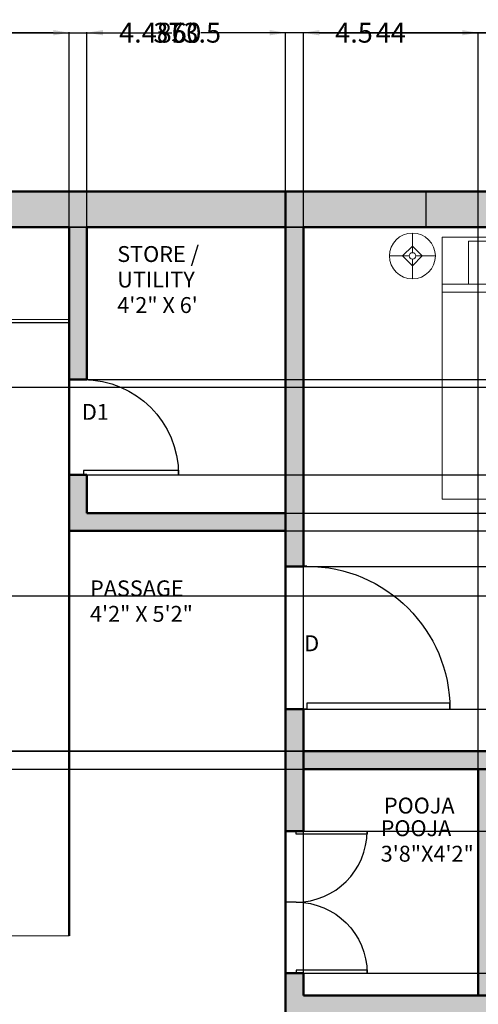
# Model space of a CAD drawing. Units: inches. Extents: x -12 to 887, y 330 to 874.
# Tile 8 of 9: x 605 to 720, y 626 to 874. Entities that reach past the tile are written whole.
import ezdxf

# ---------------------------------------------------------------- set-up
doc = ezdxf.new("R2010")
doc.units = ezdxf.units.IN
doc.header["$MEASUREMENT"] = 0
for name, color, linetype, lineweight in [('A-ANNO-DIMS', 2, 'Continuous', 18), ('A-ANNO-TEXT', 3, 'Continuous', 18), ('A-AREA-IDEN', 7, 'Continuous', 18), ('A-DOOR', 4, 'Continuous', 25), ('A-EQPM', 8, 'Continuous', 18), ('A-FLOR-FIXT', 8, 'Continuous', 18), ('A-FURN', 9, 'Continuous', 18), ('A-GLAZ', 4, 'Continuous', 25), ('A-WALL', 7, 'Continuous', 50), ('A-WALL-PATT', 5, 'Continuous', 13)]:
    doc.layers.add(name, color=color, linetype=linetype, lineweight=lineweight)
doc.styles.get("Standard").update_dxf_attribs({"font": 'arial.ttf'})
doc.dimstyles.get("Standard").update_dxf_attribs({"dimtxt": 5, "dimasz": 4, "dimexe": 0.18, "dimexo": 0.0625, "dimgap": 0.09, "dimtad": 0, "dimtih": 1, "dimtoh": 1, "dimdec": 1, "dimzin": 0, "dimdsep": 46, "dimlunit": 4, "dimtxsty": 'Standard', "dimcen": 0.09, "dimadec": 0, "dimazin": 0, "dimtfac": 1, "dimtdec": 1, "dimtofl": 0, "dimtmove": 0, "dimatfit": 3, "dimfxl": 1, "dimtolj": 1, "dimtzin": 0, "dimarcsym": 0})

# ---------------------------------------------------------------- blocks, each defined once
blk = doc.blocks.new('Refrigerator-2 door - 36 in top')
for p, q in [((0, -26.999999), (36, -26.999999)), ((11, -27.999999), (11, -28.999999)), ((12, -26.999999), (12, -28.999999)), ((13, -28.999999), (13, -27.999999)), ((11, -28.999999), (13, -28.999999))]:
    blk.add_line(p, q)
blk.add_lwpolyline([(0, -27.999999), (0, 0), (36, 0), (36, -27.999999)], close=True)
blk = doc.blocks.new('*U5')
for p, q in [((0, 0), (0, -6)), ((40, 0), (40, -6))]:
    blk.add_line(p, q)
blk.add_lwpolyline([(0, 0), (0, 40), (1.75, 40), (1.75, 0)], close=True)
blk.add_arc((0, 0), 40, 0, 90)
blk = doc.blocks.new('Bed - Queen')
for p, q in [((0, -80.00003), (0, 0)), ((0, 0), (59.99999, 0)), ((59.99999, 0), (59.99999, -80.00003)), ((7.99999, -1.2), (28.79998, -1.2)), ((7.99999, -14.4), (7.99999, -1.2)), ((28.79998, -1.2), (28.79998, -14.4)), ((31.19999, -1.2), (51.99999, -1.2)), ((31.19999, -14.4), (31.19999, -1.2)), ((51.99999, -1.2), (51.99999, -16.4)), ((0, -14.4), (44.8, -14.4)), ((59.99999, -29.6), (44.8, -14.4)), ((44.8, -14.4), (44.8, -29.6)), ((44.8, -16.8), (0, -16.8)), ((51.99999, -16.4), (46.79936, -16.4)), ((44.8, -29.6), (59.99999, -29.6)), ((59.99999, -80.00003), (0, -80.00003))]:
    blk.add_line(p, q)
blk = doc.blocks.new('Lamp - Table')
for p, q in [((0, 7), (0, 1)), ((-1, 0), (-7, 0)), ((0, 3), (-3, 0)), ((-3, 0), (0, -3)), ((3, 0), (0, 3)), ((0, -3), (3, 0)), ((1, 0), (7, 0)), ((0, -1), (0, -7))]:
    blk.add_line(p, q)
for radius in [7, 1]:
    blk.add_circle((0, 0), radius)
blk = doc.blocks.new('*D64')
at = {"layer": 'A-ANNO-DIMS', "color": 0, "lineweight": -2, "transparency": 16777216}
for p, q in [((383.99, 685.16), (873.75, 685.16)), ((873.57, 681.16), (873.57, 628.55)), ((873.57, 570.66), (873.57, 623.27)), ((383.99, 566.66), (873.75, 566.66))]:
    blk.add_line(p, q, dxfattribs=at)
at = {"layer": 'A-ANNO-DIMS', "color": 0, "transparency": 16777216}
for points in [[(872.9, 681.16), (874.24, 681.16), (873.57, 685.16)], [(872.9, 570.66), (874.24, 570.66), (873.57, 566.66)]]:
    blk.add_solid(points, dxfattribs=at)
at = {"layer": 'Defpoints', "color": 0, "transparency": 16777216}
for p in [(383.93, 685.16), (873.57, 685.16), (383.93, 566.66)]:
    blk.add_point(p, dxfattribs=at)
at = {"layer": 'A-ANNO-DIMS', "color": 0, "transparency": 16777216, "insert": (873.57, 625.91), "char_height": 5, "attachment_point": 5}
blk.add_mtext('\\A1;118.5', dxfattribs=at)
blk = doc.blocks.new('*D65')
at = {"layer": 'A-ANNO-DIMS', "color": 0, "lineweight": -2, "transparency": 16777216}
for p, q in [((873.57, 693.66), (873.57, 697.66)), ((873.57, 697.66), (877.57, 697.66)), ((383.99, 689.66), (873.75, 689.66)), ((383.99, 685.16), (873.75, 685.16)), ((873.57, 681.16), (873.57, 677.16))]:
    blk.add_line(p, q, dxfattribs=at)
at = {"layer": 'A-ANNO-DIMS', "color": 0, "transparency": 16777216}
for points in [[(872.9, 693.66), (874.24, 693.66), (873.57, 689.66)], [(872.9, 681.16), (874.24, 681.16), (873.57, 685.16)]]:
    blk.add_solid(points, dxfattribs=at)
at = {"layer": 'Defpoints', "color": 0, "transparency": 16777216}
for p in [(383.93, 689.66), (873.57, 689.66), (383.93, 685.16)]:
    blk.add_point(p, dxfattribs=at)
at = {"layer": 'A-ANNO-DIMS', "color": 0, "transparency": 16777216, "insert": (882.33, 697.66), "char_height": 5, "attachment_point": 5}
blk.add_mtext('\\A1;4.5', dxfattribs=at)
blk = doc.blocks.new('*D66')
at = {"layer": 'A-ANNO-DIMS', "color": 0, "lineweight": -2, "transparency": 16777216}
for p, q in [((383.99, 821.66), (873.75, 821.66)), ((873.57, 817.66), (873.57, 758.31)), ((873.57, 693.66), (873.57, 753.02)), ((383.99, 689.66), (873.75, 689.66))]:
    blk.add_line(p, q, dxfattribs=at)
at = {"layer": 'A-ANNO-DIMS', "color": 0, "transparency": 16777216}
for points in [[(872.9, 817.66), (874.24, 817.66), (873.57, 821.66)], [(872.9, 693.66), (874.24, 693.66), (873.57, 689.66)]]:
    blk.add_solid(points, dxfattribs=at)
at = {"layer": 'Defpoints', "color": 0, "transparency": 16777216}
for p in [(383.93, 821.66), (873.57, 821.66), (383.93, 689.66)]:
    blk.add_point(p, dxfattribs=at)
at = {"layer": 'A-ANNO-DIMS', "color": 0, "transparency": 16777216, "insert": (873.57, 755.66), "char_height": 5, "attachment_point": 5}
blk.add_mtext('\\A1;132', dxfattribs=at)
blk = doc.blocks.new('*D83')
at = {"layer": 'A-ANNO-DIMS', "color": 0, "lineweight": -2, "transparency": 16777216}
for p, q in [((460.07, 830.72), (460.07, 870.84)), ((464.07, 870.66), (638.28, 870.66)), ((829.57, 870.66), (655.36, 870.66)), ((833.57, 830.72), (833.57, 870.84))]:
    blk.add_line(p, q, dxfattribs=at)
at = {"layer": 'A-ANNO-DIMS', "color": 0, "transparency": 16777216}
for points in [[(464.07, 871.33), (464.07, 869.99), (460.07, 870.66)], [(829.57, 871.33), (829.57, 869.99), (833.57, 870.66)]]:
    blk.add_solid(points, dxfattribs=at)
at = {"layer": 'Defpoints', "color": 0, "transparency": 16777216}
for p in [(833.57, 870.66), (460.07, 830.66), (833.57, 830.66)]:
    blk.add_point(p, dxfattribs=at)
at = {"layer": 'A-ANNO-DIMS', "color": 0, "transparency": 16777216, "insert": (646.82, 870.66), "char_height": 5, "attachment_point": 5}
blk.add_mtext('\\A1;373.5', dxfattribs=at)
blk = doc.blocks.new('*D87')
at = {"layer": 'A-ANNO-DIMS', "color": 0, "lineweight": -2, "transparency": 16777216}
for p, q in [((493.07, 821.72), (493.07, 870.84)), ((497.07, 870.66), (545.32, 870.66)), ((613.08, 870.66), (564.83, 870.66)), ((617.08, 821.7), (617.08, 870.84))]:
    blk.add_line(p, q, dxfattribs=at)
at = {"layer": 'A-ANNO-DIMS', "color": 0, "transparency": 16777216}
for points in [[(497.07, 871.33), (497.07, 869.99), (493.07, 870.66)], [(613.08, 871.33), (613.08, 869.99), (617.08, 870.66)]]:
    blk.add_solid(points, dxfattribs=at)
at = {"layer": 'Defpoints', "color": 0, "transparency": 16777216}
for p in [(617.08, 870.66), (493.07, 821.66), (617.08, 821.64)]:
    blk.add_point(p, dxfattribs=at)
at = {"layer": 'A-ANNO-DIMS', "color": 0, "transparency": 16777216, "insert": (555.08, 870.66), "char_height": 5, "attachment_point": 5}
blk.add_mtext('\\A1;124.01', dxfattribs=at)
blk = doc.blocks.new('*D88')
at = {"layer": 'A-ANNO-DIMS', "color": 0, "lineweight": -2, "transparency": 16777216}
for p, q in [((613.08, 870.66), (609.08, 870.66)), ((617.08, 821.7), (617.08, 870.84)), ((621.57, 821.72), (621.57, 870.84)), ((625.57, 870.66), (629.57, 870.66))]:
    blk.add_line(p, q, dxfattribs=at)
at = {"layer": 'A-ANNO-DIMS', "color": 0, "transparency": 16777216}
for points in [[(613.08, 871.33), (613.08, 869.99), (617.08, 870.66)], [(625.57, 871.33), (625.57, 869.99), (621.57, 870.66)]]:
    blk.add_solid(points, dxfattribs=at)
at = {"layer": 'Defpoints', "color": 0, "transparency": 16777216}
for p in [(621.57, 870.66), (617.08, 821.64), (621.57, 821.66)]:
    blk.add_point(p, dxfattribs=at)
at = {"layer": 'A-ANNO-DIMS', "color": 0, "transparency": 16777216, "insert": (638.19, 870.66), "char_height": 5, "attachment_point": 5}
blk.add_mtext('\\A1;4.486', dxfattribs=at)
blk = doc.blocks.new('*D89')
at = {"layer": 'A-ANNO-DIMS', "color": 0, "lineweight": -2, "transparency": 16777216}
for p, q in [((621.57, 821.72), (621.57, 870.84)), ((625.57, 870.66), (642.91, 870.66)), ((667.57, 870.66), (650.23, 870.66)), ((671.57, 821.72), (671.57, 870.84))]:
    blk.add_line(p, q, dxfattribs=at)
at = {"layer": 'A-ANNO-DIMS', "color": 0, "transparency": 16777216}
for points in [[(625.57, 871.33), (625.57, 869.99), (621.57, 870.66)], [(667.57, 871.33), (667.57, 869.99), (671.57, 870.66)]]:
    blk.add_solid(points, dxfattribs=at)
at = {"layer": 'Defpoints', "color": 0, "transparency": 16777216}
for p in [(671.57, 870.66), (621.57, 821.66), (671.57, 821.66)]:
    blk.add_point(p, dxfattribs=at)
at = {"layer": 'A-ANNO-DIMS', "color": 0, "transparency": 16777216, "insert": (646.57, 870.66), "char_height": 5, "attachment_point": 5}
blk.add_mtext('\\A1;50', dxfattribs=at)
blk = doc.blocks.new('*D90')
at = {"layer": 'A-ANNO-DIMS', "color": 0, "lineweight": -2, "transparency": 16777216}
for p, q in [((667.57, 870.66), (663.57, 870.66)), ((671.57, 821.72), (671.57, 870.84)), ((676.07, 821.72), (676.07, 870.84)), ((680.07, 870.66), (684.07, 870.66))]:
    blk.add_line(p, q, dxfattribs=at)
at = {"layer": 'A-ANNO-DIMS', "color": 0, "transparency": 16777216}
for points in [[(667.57, 871.33), (667.57, 869.99), (671.57, 870.66)], [(680.07, 871.33), (680.07, 869.99), (676.07, 870.66)]]:
    blk.add_solid(points, dxfattribs=at)
at = {"layer": 'Defpoints', "color": 0, "transparency": 16777216}
for p in [(676.07, 870.66), (671.57, 821.66), (676.07, 821.66)]:
    blk.add_point(p, dxfattribs=at)
at = {"layer": 'A-ANNO-DIMS', "color": 0, "transparency": 16777216, "insert": (688.83, 870.66), "char_height": 5, "attachment_point": 5}
blk.add_mtext('\\A1;4.5', dxfattribs=at)
blk = doc.blocks.new('*D91')
at = {"layer": 'A-ANNO-DIMS', "color": 0, "lineweight": -2, "transparency": 16777216}
for p, q in [((676.07, 821.72), (676.07, 870.84)), ((680.07, 870.66), (733.69, 870.66)), ((798.07, 870.66), (744.44, 870.66)), ((802.07, 821.72), (802.07, 870.84))]:
    blk.add_line(p, q, dxfattribs=at)
at = {"layer": 'A-ANNO-DIMS', "color": 0, "transparency": 16777216}
for points in [[(680.07, 871.33), (680.07, 869.99), (676.07, 870.66)], [(798.07, 871.33), (798.07, 869.99), (802.07, 870.66)]]:
    blk.add_solid(points, dxfattribs=at)
at = {"layer": 'Defpoints', "color": 0, "transparency": 16777216}
for p in [(802.07, 870.66), (676.07, 821.66), (802.07, 821.66)]:
    blk.add_point(p, dxfattribs=at)
at = {"layer": 'A-ANNO-DIMS', "color": 0, "transparency": 16777216, "insert": (739.07, 870.66), "char_height": 5, "attachment_point": 5}
blk.add_mtext('\\A1;126', dxfattribs=at)
blk = doc.blocks.new('*D98')
at = {"layer": 'A-ANNO-DIMS', "color": 0, "lineweight": -2, "transparency": 16777216}
for p, q in [((460.13, 830.66), (873.75, 830.66)), ((873.57, 826.66), (873.57, 604.54)), ((873.57, 377.16), (873.57, 599.28)), ((460.13, 373.16), (873.75, 373.16))]:
    blk.add_line(p, q, dxfattribs=at)
at = {"layer": 'A-ANNO-DIMS', "color": 0, "transparency": 16777216}
for points in [[(872.9, 826.66), (874.24, 826.66), (873.57, 830.66)], [(872.9, 377.16), (874.24, 377.16), (873.57, 373.16)]]:
    blk.add_solid(points, dxfattribs=at)
at = {"layer": 'Defpoints', "color": 0, "transparency": 16777216}
for p in [(460.07, 830.66), (873.57, 830.66), (460.07, 373.16)]:
    blk.add_point(p, dxfattribs=at)
at = {"layer": 'A-ANNO-DIMS', "color": 0, "transparency": 16777216, "insert": (873.57, 601.91), "char_height": 5, "attachment_point": 5}
blk.add_mtext('\\A1;457.5', dxfattribs=at)
blk = doc.blocks.new('*D112')
at = {"layer": 'A-ANNO-DIMS', "color": 0, "lineweight": -2, "transparency": 16777216}
for p, q in [((676.01, 821.66), (1.75, 821.66)), ((1.93, 817.66), (1.93, 758.31)), ((1.93, 693.66), (1.93, 753.02)), ((676.01, 689.66), (1.75, 689.66))]:
    blk.add_line(p, q, dxfattribs=at)
at = {"layer": 'A-ANNO-DIMS', "color": 0, "transparency": 16777216}
for points in [[(1.26, 817.66), (2.59, 817.66), (1.93, 821.66)], [(1.26, 693.66), (2.59, 693.66), (1.93, 689.66)]]:
    blk.add_solid(points, dxfattribs=at)
at = {"layer": 'Defpoints', "color": 0, "transparency": 16777216}
for p in [(1.93, 821.66), (676.07, 821.66), (676.07, 689.66)]:
    blk.add_point(p, dxfattribs=at)
at = {"layer": 'A-ANNO-DIMS', "color": 0, "transparency": 16777216, "insert": (1.93, 755.66), "char_height": 5, "attachment_point": 5}
blk.add_mtext('\\A1;132', dxfattribs=at)
blk = doc.blocks.new('*D113')
at = {"layer": 'A-ANNO-DIMS', "color": 0, "lineweight": -2, "transparency": 16777216}
for p, q in [((676.07, 628.22), (676.07, 870.84)), ((680.07, 870.66), (694.31, 870.66)), ((716.07, 870.66), (701.83, 870.66)), ((720.07, 628.22), (720.07, 870.84))]:
    blk.add_line(p, q, dxfattribs=at)
at = {"layer": 'A-ANNO-DIMS', "color": 0, "transparency": 16777216}
for points in [[(680.07, 871.33), (680.07, 869.99), (676.07, 870.66)], [(716.07, 871.33), (716.07, 869.99), (720.07, 870.66)]]:
    blk.add_solid(points, dxfattribs=at)
at = {"layer": 'Defpoints', "color": 0, "transparency": 16777216}
for p in [(720.07, 870.66), (676.07, 628.16), (720.07, 628.16)]:
    blk.add_point(p, dxfattribs=at)
at = {"layer": 'A-ANNO-DIMS', "color": 0, "transparency": 16777216, "insert": (698.07, 870.66), "char_height": 5, "attachment_point": 5}
blk.add_mtext('\\A1;44', dxfattribs=at)
blk = doc.blocks.new('*D116')
at = {"layer": 'A-ANNO-DIMS', "color": 0, "lineweight": -2, "transparency": 16777216}
for p, q in [((873.57, 753.66), (873.57, 757.66)), ((621.63, 749.66), (873.75, 749.66)), ((617.13, 745.16), (873.75, 745.16)), ((873.57, 741.16), (873.57, 737.16)), ((873.57, 737.16), (869.57, 737.16))]:
    blk.add_line(p, q, dxfattribs=at)
at = {"layer": 'A-ANNO-DIMS', "color": 0, "transparency": 16777216}
for points in [[(872.9, 753.66), (874.24, 753.66), (873.57, 749.66)], [(872.9, 741.16), (874.24, 741.16), (873.57, 745.16)]]:
    blk.add_solid(points, dxfattribs=at)
at = {"layer": 'Defpoints', "color": 0, "transparency": 16777216}
for p in [(621.57, 749.66), (617.07, 745.16), (873.57, 745.16)]:
    blk.add_point(p, dxfattribs=at)
at = {"layer": 'A-ANNO-DIMS', "color": 0, "transparency": 16777216, "insert": (864.81, 737.16), "char_height": 5, "attachment_point": 5}
blk.add_mtext('\\A1;4.5', dxfattribs=at)
blk = doc.blocks.new('*D117')
at = {"layer": 'A-ANNO-DIMS', "color": 0, "lineweight": -2, "transparency": 16777216}
for p, q in [((621.63, 821.66), (873.75, 821.66)), ((873.57, 817.66), (873.57, 788.26)), ((873.57, 753.66), (873.57, 783.06)), ((621.63, 749.66), (873.75, 749.66))]:
    blk.add_line(p, q, dxfattribs=at)
at = {"layer": 'A-ANNO-DIMS', "color": 0, "transparency": 16777216}
for points in [[(872.9, 817.66), (874.24, 817.66), (873.57, 821.66)], [(872.9, 753.66), (874.24, 753.66), (873.57, 749.66)]]:
    blk.add_solid(points, dxfattribs=at)
at = {"layer": 'Defpoints', "color": 0, "transparency": 16777216}
for p in [(621.57, 821.66), (873.57, 821.66), (621.57, 749.66)]:
    blk.add_point(p, dxfattribs=at)
at = {"layer": 'A-ANNO-DIMS', "color": 0, "transparency": 16777216, "insert": (873.57, 785.66), "char_height": 5, "attachment_point": 5}
blk.add_mtext('\\A1;72', dxfattribs=at)
blk = doc.blocks.new('*D122')
at = {"layer": 'A-ANNO-DIMS', "color": 0, "lineweight": -2, "transparency": 16777216}
for p, q in [((671.63, 736.22), (873.75, 736.22)), ((873.57, 732.22), (873.57, 720.87)), ((873.57, 704.22), (873.57, 715.58)), ((671.63, 700.22), (873.75, 700.22))]:
    blk.add_line(p, q, dxfattribs=at)
at = {"layer": 'A-ANNO-DIMS', "color": 0, "transparency": 16777216}
for points in [[(872.9, 732.22), (874.24, 732.22), (873.57, 736.22)], [(872.9, 704.22), (874.24, 704.22), (873.57, 700.22)]]:
    blk.add_solid(points, dxfattribs=at)
at = {"layer": 'Defpoints', "color": 0, "transparency": 16777216}
for p in [(671.57, 736.22), (671.57, 700.22), (873.57, 700.22)]:
    blk.add_point(p, dxfattribs=at)
at = {"layer": 'A-ANNO-DIMS', "color": 0, "transparency": 16777216, "insert": (873.57, 718.22), "char_height": 5, "attachment_point": 5}
blk.add_mtext('\\A1;36', dxfattribs=at)
blk = doc.blocks.new('*D123')
at = {"layer": 'A-ANNO-DIMS', "color": 0, "lineweight": -2, "transparency": 16777216}
for p, q in [((617.13, 783.29), (873.75, 783.29)), ((873.57, 779.29), (873.57, 773.94)), ((873.57, 763.31), (873.57, 768.65)), ((617.13, 759.31), (873.75, 759.31))]:
    blk.add_line(p, q, dxfattribs=at)
at = {"layer": 'A-ANNO-DIMS', "color": 0, "transparency": 16777216}
for points in [[(872.9, 779.29), (874.24, 779.29), (873.57, 783.29)], [(872.9, 763.31), (874.24, 763.31), (873.57, 759.31)]]:
    blk.add_solid(points, dxfattribs=at)
at = {"layer": 'Defpoints', "color": 0, "transparency": 16777216}
for p in [(617.07, 783.29), (617.07, 759.31), (873.57, 759.31)]:
    blk.add_point(p, dxfattribs=at)
at = {"layer": 'A-ANNO-DIMS', "color": 0, "transparency": 16777216, "insert": (873.57, 771.3), "char_height": 5, "attachment_point": 5}
blk.add_mtext('\\A1;23.98', dxfattribs=at)
blk = doc.blocks.new('*D127')
at = {"layer": 'A-ANNO-DIMS', "color": 0, "lineweight": -2, "transparency": 16777216}
for p, q in [((671.63, 669.51), (873.75, 669.51)), ((873.57, 665.51), (873.57, 654.28)), ((873.57, 637.77), (873.57, 648.99)), ((671.63, 633.77), (873.75, 633.77))]:
    blk.add_line(p, q, dxfattribs=at)
at = {"layer": 'A-ANNO-DIMS', "color": 0, "transparency": 16777216}
for points in [[(872.9, 665.51), (874.24, 665.51), (873.57, 669.51)], [(872.9, 637.77), (874.24, 637.77), (873.57, 633.77)]]:
    blk.add_solid(points, dxfattribs=at)
at = {"layer": 'Defpoints', "color": 0, "transparency": 16777216}
for p in [(671.57, 669.51), (671.57, 633.77), (873.57, 633.77)]:
    blk.add_point(p, dxfattribs=at)
at = {"layer": 'A-ANNO-DIMS', "color": 0, "transparency": 16777216, "insert": (873.57, 651.64), "char_height": 5, "attachment_point": 5}
blk.add_mtext('\\A1;35.745', dxfattribs=at)
blk = doc.blocks.new('*D128')
at = {"layer": 'A-ANNO-DIMS', "color": 0, "lineweight": -2, "transparency": 16777216}
for p, q in [((488.63, 781.36), (873.75, 781.36)), ((873.57, 777.36), (873.57, 757.74)), ((873.57, 732.83), (873.57, 752.45)), ((488.63, 728.83), (873.75, 728.83))]:
    blk.add_line(p, q, dxfattribs=at)
at = {"layer": 'A-ANNO-DIMS', "color": 0, "transparency": 16777216}
for points in [[(872.9, 777.36), (874.24, 777.36), (873.57, 781.36)], [(872.9, 732.83), (874.24, 732.83), (873.57, 728.83)]]:
    blk.add_solid(points, dxfattribs=at)
at = {"layer": 'Defpoints', "color": 0, "transparency": 16777216}
for p in [(488.57, 781.36), (488.57, 728.83), (873.57, 728.83)]:
    blk.add_point(p, dxfattribs=at)
at = {"layer": 'A-ANNO-DIMS', "color": 0, "transparency": 16777216, "insert": (873.57, 755.1), "char_height": 5, "attachment_point": 5}
blk.add_mtext('\\A1;52.54', dxfattribs=at)

msp = doc.modelspace()

# ---------------------------------------------------------------- hatches: boundary and pattern name
at = {"layer": 'A-WALL-PATT'}
h = msp.add_hatch(color=256, dxfattribs=at)
h.dxf.hatch_style = 1
h.paths.add_polyline_path([(94.575, 830.6611), (67.3199, 830.6611), (67.3199, 821.6611), (70.4263, 821.6611), (79.4263, 821.6611), (94.575, 821.6611)])
h.paths.add_polyline_path([(288.8031, 830.6611), (257.9263, 830.6611), (253.4263, 830.6611), (253.4263, 821.6611), (288.8031, 821.6611)])
h.paths.add_polyline_path([(74.9263, 696.9265), (70.4263, 696.9265), (70.4263, 678.4656), (74.9263, 678.4656)])
h.paths.add_polyline_path([(74.9263, 584.8756), (70.4263, 584.8756), (70.4263, 562.1611), (74.9263, 562.1611)])
h.paths.add_polyline_path([(135.5357, 566.6611), (122.6994, 566.6611), (122.6994, 562.1611), (135.5357, 562.1611)])
h.paths.add_polyline_path([(257.9263, 579.1607), (253.4263, 579.1607), (253.4263, 562.1611), (257.9263, 562.1611)])
h.paths.add_polyline_path([(272.0195, 454.1611), (254.2006, 454.1611), (254.2006, 450.1611), (272.0195, 450.1611)])
h.paths.add_polyline_path([(392.9263, 454.1611), (374.959, 454.1611), (374.959, 450.1611), (383.9263, 450.1611), (392.9263, 450.1611)])
h.paths.add_polyline_path([(493.0683, 466.4171), (488.5683, 466.4171), (488.5683, 450.1611), (493.0683, 450.1611)])
h.paths.add_polyline_path([(568.6302, 454.1611), (555.938, 454.1611), (555.938, 450.1611), (568.6302, 450.1611)])
h.paths.add_polyline_path([(493.0683, 594.9471), (488.5683, 594.9471), (488.5683, 569.5862), (493.0683, 569.5862)])
h.paths.add_polyline_path([(690.1615, 454.1611), (672.3426, 454.1611), (672.3426, 450.1611), (690.1615, 450.1611)])
h.paths.add_polyline_path([(811.0683, 454.1611), (793.101, 454.1611), (793.101, 450.1611), (802.0683, 450.1611), (811.0683, 450.1611)])
h.paths.add_polyline_path([(811.0683, 578.3606), (802.0683, 578.3606), (802.0683, 566.6611), (802.0683, 553.5254), (811.0683, 553.5254)])
h.paths.add_polyline_path([(811.0683, 701.6611), (802.0683, 701.6611), (802.0683, 689.9616), (802.0683, 676.8259), (811.0683, 676.8259)])
h.paths.add_polyline_path([(811.0683, 830.6611), (782.165, 830.6611), (782.165, 821.6611), (802.0683, 821.6611), (811.0683, 821.6611)])
h.paths.add_polyline_path([(706.9451, 830.6611), (671.5683, 830.6611), (671.5683, 821.6611), (706.9451, 821.6611)])
h.paths.add_polyline_path([(512.717, 830.6611), (485.4619, 830.6611), (485.4619, 821.6611), (488.5683, 821.6611), (512.717, 821.6611)])
h.paths.add_polyline_path([(392.9263, 697.8668), (383.9263, 697.8668), (383.9263, 689.6611), (383.9263, 676.5034), (392.9263, 676.5034)])
h.paths.add_polyline_path([(392.9263, 830.6611), (364.023, 830.6611), (364.023, 821.7357), (392.9263, 821.7357)])
h.paths.add_polyline_path([(392.9263, 619.0434), (383.9263, 619.0434), (383.9263, 588.7499), (392.9263, 588.7499)])
h.paths.add_polyline_path([(392.9263, 578.3606), (383.9263, 578.3606), (383.9263, 566.6611), (383.9263, 553.5254), (392.9263, 553.5254)])
h.paths.add_polyline_path([(257.9263, 699.8547), (253.4263, 699.8547), (253.4263, 697.1611), (253.4263, 677.338), (257.9263, 677.338)])
h.paths.add_polyline_path([(493.0683, 714.3785), (488.5683, 714.3785), (488.5683, 689.6611), (493.0683, 689.6611)])
h.paths.add_polyline_path([(74.9263, 491.4191), (70.4263, 491.4191), (70.4263, 480.7097), (74.9263, 480.7097)])
h = msp.add_hatch(color=256, dxfattribs=at)
h.dxf.hatch_style = 1
h.paths.add_polyline_path([(671.5683, 830.6611), (512.717, 830.6611), (512.717, 821.6611), (617.0825, 821.6611), (617.0825, 797.5825), (617.0787, 783.3094), (621.5683, 783.3094), (621.5683, 821.6611), (671.5683, 821.6611)], flags=17)
h.paths.add_polyline_path([(833.5683, 830.6611), (811.0683, 830.6611), (811.0683, 821.6611), (829.0683, 821.6611), (829.0683, 701.6611), (829.0683, 382.1611), (811.0683, 382.1611), (811.0683, 450.1611), (802.0683, 450.1611), (802.0683, 382.1611), (671.5683, 382.1611), (464.5683, 382.1611), (464.5683, 821.6611), (460.0683, 821.6611), (460.0683, 373.1611), (671.5683, 373.1611), (833.5683, 373.1611)])
h.paths.add_polyline_path([(493.0683, 728.8273), (488.5683, 728.8273), (488.5683, 714.3785), (493.0683, 714.3785)], flags=17)
h.paths.add_polyline_path([(493.0683, 821.6611), (488.5683, 821.6611), (488.5683, 781.3634), (493.0683, 781.3634)], flags=17)
h = msp.add_hatch(color=256, dxfattribs=at)
h.dxf.hatch_style = 1
h.paths.add_polyline_path([(671.5683, 749.6611), (621.5683, 749.6611), (621.5683, 759.3094), (620.6653, 759.3094), (617.0683, 759.3094), (617.0683, 745.1611), (671.5683, 745.1611)])
h.paths.add_polyline_path([(676.0683, 821.6611), (671.5683, 821.6611), (671.5683, 736.2424), (676.0683, 736.2424)])
h.paths.add_polyline_path([(782.165, 830.6611), (706.9451, 830.6611), (706.9451, 821.6611), (782.165, 821.6611)])
h.paths.add_polyline_path([(811.0683, 553.5254), (802.0683, 553.5254), (802.0683, 507.4529), (802.0683, 454.1611), (811.0683, 454.1611)])
h.paths.add_polyline_path([(793.101, 454.1611), (690.1615, 454.1611), (690.1615, 450.1611), (793.101, 450.1611)])
h.paths.add_polyline_path([(672.3426, 454.1611), (656.7304, 454.1611), (656.7304, 450.1611), (672.3426, 450.1611)])
h.paths.add_polyline_path([(582.6585, 454.1611), (568.6302, 454.1611), (568.6302, 450.1611), (582.6585, 450.1611)])
h.paths.add_polyline_path([(555.938, 454.1611), (554.2565, 454.1611), (554.2565, 452.8628), (554.2565, 450.1611), (555.938, 450.1611)])
h.paths.add_polyline_path([(518.2335, 452.8628), (518.2335, 454.1611), (493.0683, 454.1611), (493.0683, 450.1611), (518.2335, 450.1611)])
h.paths.add_polyline_path([(493.0683, 450.1611), (488.5683, 450.1611), (488.5683, 382.1611), (493.0683, 382.1611)])
h.paths.add_polyline_path([(493.0683, 492.3446), (488.5683, 492.3446), (488.5683, 466.4171), (493.0683, 466.4171)])
h.paths.add_polyline_path([(493.0683, 569.5862), (488.5683, 569.5862), (488.5683, 557.2595), (493.0683, 557.2595)])
h.paths.add_polyline_path([(493.0683, 689.6611), (488.5683, 689.6611), (488.5683, 594.9471), (493.0683, 594.9471)])
h.paths.add_polyline_path([(676.0683, 700.2227), (671.5683, 700.2227), (671.5683, 669.5589), (676.0683, 669.5589)])
h.paths.add_polyline_path([(739.0683, 689.6611), (676.0683, 689.6611), (676.0683, 685.1611), (739.0683, 685.1611)])
h.paths.add_polyline_path([(802.0683, 689.6611), (763.0683, 689.6611), (763.0683, 686.0698), (763.0683, 685.1611), (802.0683, 685.1611)])
h.paths.add_polyline_path([(811.0683, 821.6611), (802.0683, 821.6611), (802.0683, 756.0738), (811.0683, 756.0738)])
h.paths.add_polyline_path([(811.0683, 707.8935), (802.0683, 707.8935), (802.0683, 701.6611), (811.0683, 701.6611)])
h.paths.add_polyline_path([(811.0683, 676.8259), (802.0683, 676.8259), (802.0683, 628.1611), (730.0683, 628.1611), (730.0683, 623.6611), (802.0683, 623.6611), (802.0683, 578.3606), (811.0683, 578.3606)])
h.paths.add_polyline_path([(730.0683, 685.1611), (726.0683, 685.1611), (726.0683, 628.1611), (730.0683, 628.1611)])
h.paths.add_polyline_path([(724.0683, 685.1611), (720.0683, 685.1611), (720.0683, 628.1611), (724.0683, 628.1611)])
h.paths.add_polyline_path([(726.0683, 628.1611), (676.0683, 628.1611), (676.0683, 633.7662), (674.2492, 633.7662), (671.5683, 633.7662), (671.5683, 623.6611), (726.0683, 623.6611)])
h.paths.add_polyline_path([(730.0683, 628.1611), (726.0683, 628.1611), (726.0683, 623.6611), (730.0683, 623.6611)])
h.paths.add_polyline_path([(730.0683, 623.6611), (726.0683, 623.6611), (726.0683, 595.3822), (729.6731, 595.3822, -0.00411226), (730.0683, 595.379)])
h.paths.add_polyline_path([(802.0683, 564.6611), (730.0683, 564.6611), (730.0683, 571.3507), (729.6731, 571.3507), (726.0683, 571.3507), (726.0683, 564.6611), (718.522, 564.6611), (718.522, 560.1611), (802.0683, 560.1611)])
h.paths.add_polyline_path([(676.0683, 580.4772), (671.5683, 580.4772), (671.5683, 560.1611), (676.0683, 560.1611)])
h.paths.add_polyline_path([(682.5176, 564.6611), (676.0683, 564.6611), (676.0683, 560.1611), (682.5176, 560.1611)])
h.paths.add_polyline_path([(676.0683, 560.1611), (671.5683, 560.1611), (671.5683, 454.1611), (672.3426, 454.1611), (676.0683, 454.1611)])

# ---------------------------------------------------------------- linework, layer by layer
at = {"layer": 'A-FLOR-FIXT'}
for p, q in [((521.5683, 797.6611), (617.0683, 797.6611)), ((493.0683, 643.1611), (617.0683, 643.1611))]:
    msp.add_line(p, q, dxfattribs=at)
at = {"layer": 'A-GLAZ'}
msp.add_lwpolyline([(671.5683, 821.6611), (671.5683, 830.6611), (706.9451, 830.6611), (706.9451, 821.6611), (671.5683, 821.6611)], dxfattribs=at)
at = {"layer": 'A-WALL'}
for p, q in [((460.0683, 830.6611), (671.5683, 830.6611)), ((671.5683, 830.6611), (671.5683, 584.9963)), ((671.5683, 830.6611), (676.0683, 830.6611)), ((676.0683, 830.6611), (833.5683, 830.6611)), ((497.5683, 821.6611), (617.0683, 821.6611)), ((617.0683, 821.6611), (617.0683, 745.1611)), ((621.5683, 821.6611), (621.5683, 783.3094)), ((621.5683, 821.6611), (671.5683, 821.6611)), ((676.0683, 821.6611), (676.0683, 736.2227)), ((676.0683, 821.6611), (811.0683, 821.6611)), ((621.5683, 783.3094), (617.0683, 783.3094)), ((617.0683, 759.3094), (621.5683, 759.3094)), ((621.5683, 759.3094), (621.5683, 749.6611)), ((621.5683, 749.6611), (671.5683, 749.6611)), ((617.0683, 745.1611), (671.5683, 745.1611)), ((617.0683, 745.1611), (617.0683, 643.1611)), ((671.5683, 736.2227), (676.0683, 736.2227)), ((676.0683, 700.2227), (671.5683, 700.2227)), ((676.0683, 700.2227), (676.0683, 669.5589)), ((676.0683, 689.6611), (802.0683, 689.6611)), ((676.0683, 685.1611), (739.0683, 685.1611)), ((720.0683, 685.1611), (720.0683, 628.1611)), ((676.0683, 669.5589), (671.5683, 669.5589)), ((671.5683, 633.7662), (676.0683, 633.7662)), ((676.0683, 633.7662), (676.0683, 628.1611)), ((676.0683, 628.1611), (802.0683, 628.1611))]:
    msp.add_line(p, q, dxfattribs=at)

# ---------------------------------------------------------------- block references
at = {"layer": 'A-DOOR', "rotation": 270}
for p, xscale, yscale, zscale in [((620.6653, 759.3094), -0.5994880856815563, 0.5994880856815563, 0.5994880856815563), ((676.9713, 700.2227), -0.9004920544918665, 0.9004920544918665, 0.9004920544918665), ((674.2492, 669.5108), 0.4468078227487168, 0.4468078227487168, 0.4468078227487168), ((674.2492, 633.7662), -0.4468078227487168, 0.4468078227487168, 0.4468078227487168)]:
    msp.add_blockref('*U5', p, dxfattribs=dict(at, xscale=xscale, yscale=yscale, zscale=zscale))
at = {"layer": 'A-EQPM', "xscale": 0.8591090410497297, "yscale": 0.8591090410497297, "zscale": 0.8591090410497297}
msp.add_blockref('Refrigerator-2 door - 36 in top', (586.1546, 821.6375), dxfattribs=at)
at = {"layer": 'A-FURN', "xscale": 0.8252380322911079, "yscale": 0.8252380322911079, "zscale": 0.8252380322911079}
for name, p in [('Lamp - Table', (703.5396, 814.4212)), ('Bed - Queen', (711.048, 819.1735))]:
    msp.add_blockref(name, p, dxfattribs=at)

# ---------------------------------------------------------------- texts
at = {"layer": 'A-ANNO-TEXT'}
for s, p in [('D1', (620.3085, 773.144)), ('D', (676.2988, 714.8537))]:
    msp.add_text(s, height=4, dxfattribs=at).set_placement(p)
at = {"layer": 'A-AREA-IDEN'}
for s, p in [('STORE /', (629.1963, 812.9118)), ('UTILITY', (629.1963, 806.4862)), ('4\'2" X 6\'', (629.1963, 800.0605)), ('PASSAGE', (622.3475, 728.6952)), ('4\'2" X 5\'2"', (622.3475, 722.2695)), ('POOJA', (696.3634, 673.9732)), ('POOJA ', (695.5482, 668.2705)), ('3\'8"X4\'2"', (695.5482, 661.8449))]:
    msp.add_text(s, height=4, dxfattribs=at).set_placement(p)

# ---------------------------------------------------------------- dimensions: what is measured, and where the dimension line sits
at = {"layer": 'A-ANNO-DIMS'}
for base, p1, p2, override, picture, middle in [((833.5683, 870.6611), (460.0683, 830.6611), (833.5683, 830.6611), {"dimdec": 1, "dimlfac": 1, "dimrnd": 0, "dimzin": 0, "dimdsep": 46, "dimlunit": 2}, '*D83', (646.8183, 870.6611)), ((617.0825, 870.6611), (493.0683, 821.6611), (617.0825, 821.6375), {"dimdec": 2, "dimlfac": 1, "dimrnd": 0, "dimzin": 0, "dimdsep": 46, "dimlunit": 2}, '*D87', (555.0754, 870.6611)), ((621.5683, 870.6611), (617.0825, 821.6375), (621.5683, 821.6611), {"dimdec": 3, "dimlfac": 1, "dimrnd": 0, "dimzin": 0, "dimdsep": 46, "dimlunit": 2}, '*D88', (638.1935, 870.6611)), ((671.5683, 870.6611), (621.5683, 821.6611), (671.5683, 821.6611), {"dimdec": 0, "dimlfac": 1, "dimrnd": 0, "dimzin": 0, "dimdsep": 46, "dimlunit": 2}, '*D89', (646.5683, 870.6611)), ((676.0683, 870.6611), (671.5683, 821.6611), (676.0683, 821.6611), {"dimdec": 1, "dimlfac": 1, "dimrnd": 0, "dimzin": 0, "dimdsep": 46, "dimlunit": 2}, '*D90', (688.8292, 870.6611)), ((802.0683, 870.6611), (676.0683, 821.6611), (802.0683, 821.6611), {"dimdec": 0, "dimlfac": 1, "dimrnd": 0, "dimzin": 0, "dimdsep": 46, "dimlunit": 2}, '*D91', (739.0683, 870.6611)), ((720.0683, 870.6611), (676.0683, 628.1611), (720.0683, 628.1611), {"dimdec": 0, "dimlfac": 1, "dimrnd": 0, "dimzin": 0, "dimdsep": 46, "dimlunit": 2}, '*D113', (698.0683, 870.6611))]:
    dim = msp.add_linear_dim(base=base, p1=p1, p2=p2, dimstyle='Standard', override=override, dxfattribs=at)
    dim.commit()
    dim.dimension.update_dxf_attribs({"geometry": picture, "text_midpoint": middle})
for base, p1, p2, override, picture, middle in [((873.5683, 830.6611), (460.0683, 373.1611), (460.0683, 830.6611), {"dimdec": 1, "dimlfac": 1, "dimrnd": 0, "dimzin": 0, "dimdsep": 46, "dimlunit": 2}, '*D98', (873.5683, 601.9111)), ((1.9263, 821.6611), (676.0683, 689.6611), (676.0683, 821.6611), {"dimdec": 0, "dimlfac": 1, "dimrnd": 0, "dimzin": 0, "dimdsep": 46, "dimlunit": 2}, '*D112', (1.9263, 755.6611)), ((873.5683, 821.6611), (383.9263, 689.6611), (383.9263, 821.6611), {"dimdec": 0, "dimlfac": 1, "dimrnd": 0, "dimzin": 0, "dimdsep": 46, "dimlunit": 2}, '*D66', (873.5683, 755.6611)), ((873.5683, 821.6611), (621.5683, 749.6611), (621.5683, 821.6611), {"dimdec": 0, "dimlfac": 1, "dimrnd": 0, "dimzin": 0, "dimdsep": 46, "dimlunit": 2}, '*D117', (873.5683, 785.6611)), ((873.5683, 728.8273), (488.5683, 781.3634), (488.5683, 728.8273), {"dimdec": 2, "dimlfac": 1, "dimrnd": 0, "dimzin": 0, "dimdsep": 46, "dimlunit": 2}, '*D128', (873.5683, 755.0953)), ((873.5683, 759.3094), (617.0683, 783.289), (617.0683, 759.3094), {"dimdec": 2, "dimlfac": 1, "dimrnd": 0, "dimzin": 0, "dimdsep": 46, "dimlunit": 2}, '*D123', (873.5683, 771.2992)), ((873.5683, 745.1611), (621.5683, 749.6611), (617.0683, 745.1611), {"dimdec": 1, "dimlfac": 1, "dimrnd": 0, "dimzin": 0, "dimdsep": 46, "dimlunit": 2}, '*D116', (864.8075, 737.1611)), ((873.5683, 700.2227), (671.5683, 736.2227), (671.5683, 700.2227), {"dimdec": 0, "dimlfac": 1, "dimrnd": 0, "dimzin": 0, "dimdsep": 46, "dimlunit": 2}, '*D122', (873.5683, 718.2227)), ((873.5683, 689.6611), (383.9263, 685.1611), (383.9263, 689.6611), {"dimdec": 1, "dimlfac": 1, "dimrnd": 0, "dimzin": 0, "dimdsep": 46, "dimlunit": 2}, '*D65', (882.3292, 697.6611)), ((873.5683, 685.1611), (383.9263, 566.6611), (383.9263, 685.1611), {"dimdec": 1, "dimlfac": 1, "dimrnd": 0, "dimzin": 0, "dimdsep": 46, "dimlunit": 2}, '*D64', (873.5683, 625.9111)), ((873.5683, 633.7662), (671.5683, 669.5108), (671.5683, 633.7662), {"dimdec": 3, "dimlfac": 1, "dimrnd": 0, "dimzin": 0, "dimdsep": 46, "dimlunit": 2}, '*D127', (873.5683, 651.6385))]:
    dim = msp.add_linear_dim(base=base, p1=p1, p2=p2, angle=90, dimstyle='Standard', override=override, dxfattribs=at)
    dim.commit()
    dim.dimension.update_dxf_attribs({"geometry": picture, "text_midpoint": middle})

doc.saveas('drawing.dxf')
